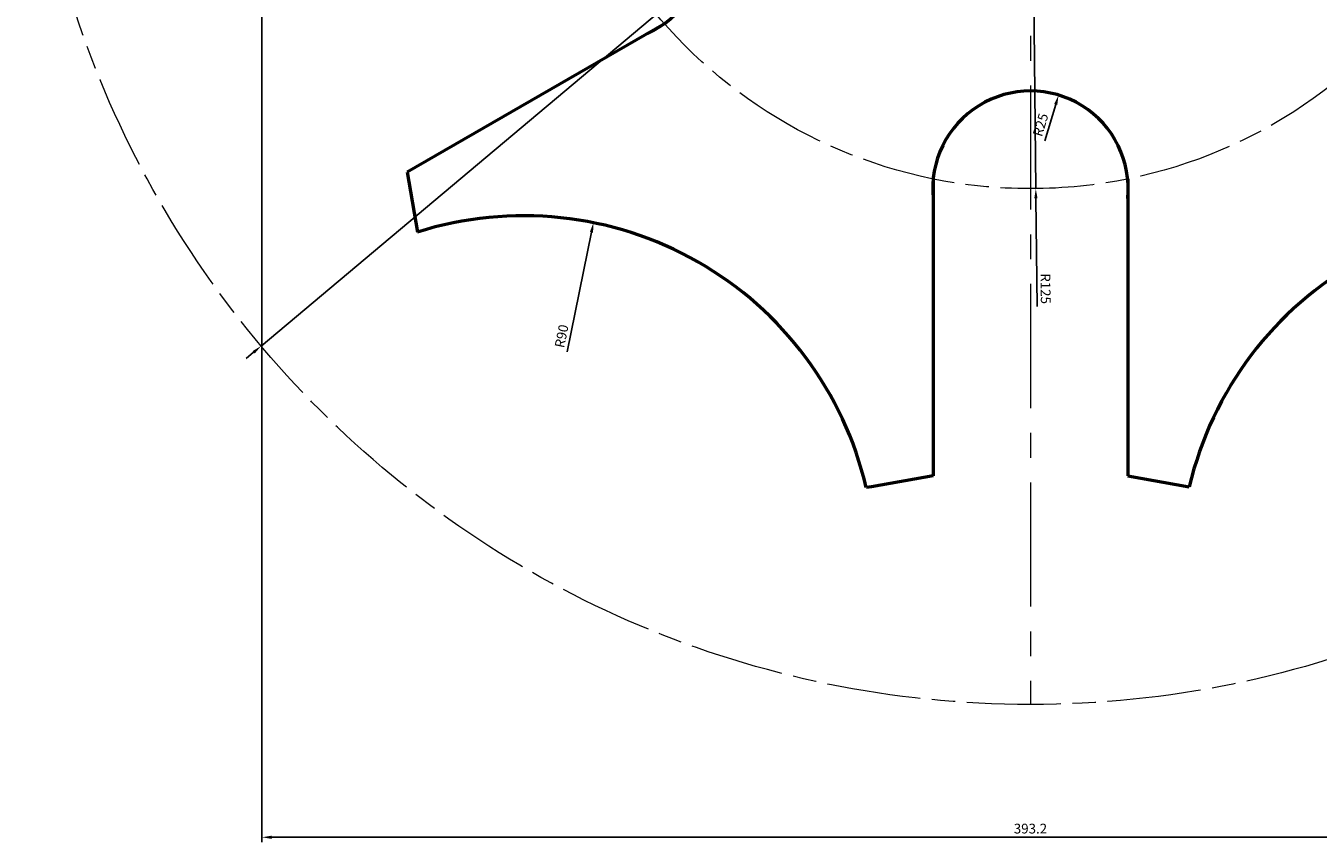
# Model space of a CAD drawing. Units: millimetres. Extents: x 1944 to 2645, y 1235 to 1798.
# Tile 1 of 3: x 2069 to 2400, y 1235 to 1444. Entities that reach past the tile are written whole.
import ezdxf

# ---------------------------------------------------------------- set-up
doc = ezdxf.new("R2010")
doc.units = ezdxf.units.MM
doc.linetypes.add('ACAD_ISO08W100', pattern=[36, 24, -3, 6, -3])
doc.linetypes.add('CENTER', pattern=[50.8, 31.75, -6.35, 6.35, -6.35])
for name, color, linetype, lineweight in [('M-CNTR', 4, 'CENTER', 18), ('M-CONS', 8, 'ACAD_ISO08W100', 18), ('M-DIMS', 2, 'Continuous', 25), ('M-OUTL', 7, 'Continuous', 50)]:
    doc.layers.add(name, color=color, linetype=linetype, lineweight=lineweight)
doc.styles.get("Standard").update_dxf_attribs({"font": 'arial.ttf'})
doc.dimstyles.new('ISO-25', dxfattribs={"dimtxt": 2.5, "dimasz": 2.5, "dimexe": 1.25, "dimexo": 0.625, "dimtad": 1, "dimdec": 1, "dimdsep": 46, "dimtxsty": 'Standard', "dimcen": 2.5, "dimadec": 0, "dimazin": 0, "dimtfac": 1, "dimtdec": 1, "dimtmove": 0, "dimatfit": 3, "dimfxl": 1, "dimarcsym": 0})

# ---------------------------------------------------------------- blocks, each defined once
blk = doc.blocks.new('*D3')
at = {"layer": 'Defpoints', "color": 0, "lineweight": 100, "transparency": 16777216}
for p in [(2333.34, 1426.64), (2326.15, 1402.69)]:
    blk.add_point(p, dxfattribs=at)
at = {"layer": 'M-DIMS', "color": 0, "lineweight": -2, "transparency": 16777216}
blk.add_line((2329.82, 1414.91), (2332.62, 1424.24), dxfattribs=at)
at = {"layer": 'M-DIMS', "color": 0, "lineweight": 100, "transparency": 16777216}
blk.add_solid([(2332.22, 1424.36), (2333.02, 1424.12), (2333.34, 1426.64)], dxfattribs=at)
at = {"layer": 'M-DIMS', "color": 0, "transparency": 16777216, "insert": (2329.04, 1418.93), "char_height": 2.5, "attachment_point": 5, "rotation": 73.2857}
blk.add_mtext('R25', dxfattribs=at)
blk = doc.blocks.new('*D6')
at = {"layer": 'Defpoints', "color": 0, "lineweight": 100, "transparency": 16777216}
for p in [(2326.15, 1527.69), (2327.52, 1402.7)]:
    blk.add_point(p, dxfattribs=at)
at = {"layer": 'M-DIMS', "color": 0, "lineweight": -2, "transparency": 16777216}
for p, q in [((2326.15, 1527.69), (2327.52, 1402.7)), ((2327.85, 1372.49), (2327.55, 1400.2))]:
    blk.add_line(p, q, dxfattribs=at)
at = {"layer": 'M-DIMS', "color": 0, "lineweight": 100, "transparency": 16777216}
blk.add_solid([(2327.96, 1400.2), (2327.13, 1400.19), (2327.52, 1402.7)], dxfattribs=at)
at = {"layer": 'M-DIMS', "color": 0, "transparency": 16777216, "insert": (2329.7, 1377.1), "char_height": 2.5, "attachment_point": 5, "rotation": 270.6275}
blk.add_mtext('R125', dxfattribs=at)
blk = doc.blocks.new('*D7')
at = {"layer": 'Defpoints', "color": 0, "lineweight": 100, "transparency": 16777216}
for p in [(2214.35, 1393.97), (2196.48, 1305.76)]:
    blk.add_point(p, dxfattribs=at)
at = {"layer": 'M-DIMS', "color": 0, "lineweight": -2, "transparency": 16777216}
blk.add_line((2207.66, 1360.97), (2213.85, 1391.52), dxfattribs=at)
at = {"layer": 'M-DIMS', "color": 0, "lineweight": 100, "transparency": 16777216}
blk.add_solid([(2213.44, 1391.6), (2214.26, 1391.44), (2214.35, 1393.97)], dxfattribs=at)
at = {"layer": 'M-DIMS', "color": 0, "transparency": 16777216, "insert": (2206.52, 1364.88), "char_height": 2.5, "attachment_point": 5, "rotation": 78.5527}
blk.add_mtext('R90', dxfattribs=at)
blk = doc.blocks.new('*D13')
at = {"layer": 'Defpoints', "color": 0, "lineweight": 100, "transparency": 16777216}
for p in [(2160.02, 1723.78), (2492.28, 1331.61)]:
    blk.add_point(p, dxfattribs=at)
at = {"layer": 'M-DIMS', "color": 0, "lineweight": -2, "transparency": 16777216}
blk.add_line((2467.27, 1361.13), (2490.67, 1333.51), dxfattribs=at)
at = {"layer": 'M-DIMS', "color": 0, "lineweight": 100, "transparency": 16777216}
blk.add_solid([(2490.98, 1333.78), (2490.35, 1333.24), (2492.28, 1331.61)], dxfattribs=at)
at = {"layer": 'M-DIMS', "color": 0, "transparency": 16777216, "insert": (2471.84, 1358.79), "char_height": 2.5, "attachment_point": 5, "rotation": 310.2727}
blk.add_mtext('∅514', dxfattribs=at)
blk = doc.blocks.new('GENEVA-RADIAL-SLOT-R25')
for p, q in [((0.13, 76), (0.13, 0)), ((49.87, 76), (49.87, 0))]:
    blk.add_line(p, q)
blk.add_arc((25, 73.5), 25, 354.2608, 185.7392)
blk = doc.blocks.new('*D17')
at = {"layer": 'Defpoints', "color": 0, "lineweight": 100, "transparency": 16777216}
for p in [(2129.55, 1460.27), (2522.75, 1460.27), (2522.75, 1236.69)]:
    blk.add_point(p, dxfattribs=at)
at = {"layer": 'M-DIMS', "color": 0, "lineweight": -2, "transparency": 16777216}
for p, q in [((2129.55, 1459.64), (2129.55, 1235.44)), ((2522.75, 1459.64), (2522.75, 1235.44)), ((2132.05, 1236.69), (2520.25, 1236.69))]:
    blk.add_line(p, q, dxfattribs=at)
at = {"layer": 'M-DIMS', "color": 0, "lineweight": 100, "transparency": 16777216}
for points in [[(2132.05, 1237.11), (2132.05, 1236.27), (2129.55, 1236.69)], [(2520.25, 1237.11), (2520.25, 1236.27), (2522.75, 1236.69)]]:
    blk.add_solid(points, dxfattribs=at)
at = {"layer": 'M-DIMS', "color": 0, "transparency": 16777216, "insert": (2326.15, 1238.59), "char_height": 2.5, "attachment_point": 5}
blk.add_mtext('393.2', dxfattribs=at)
blk = doc.blocks.new('*D18')
at = {"layer": 'Defpoints', "color": 0, "lineweight": 100, "transparency": 16777216}
for p in [(2522.96, 1692.97), (2129.34, 1362.42)]:
    blk.add_point(p, dxfattribs=at)
at = {"layer": 'M-DIMS', "color": 0, "lineweight": -2, "transparency": 16777216}
for p, q in [((2644.67, 1795.18), (2524.87, 1694.57)), ((2129.34, 1362.42), (2522.96, 1692.97)), ((2127.43, 1360.81), (2125.51, 1359.2))]:
    blk.add_line(p, q, dxfattribs=at)
at = {"layer": 'M-DIMS', "color": 0, "lineweight": 100, "transparency": 16777216}
for points in [[(2524.61, 1694.89), (2525.14, 1694.25), (2522.96, 1692.97)], [(2127.16, 1361.13), (2127.69, 1360.49), (2129.34, 1362.42)]]:
    blk.add_solid(points, dxfattribs=at)
at = {"layer": 'M-DIMS', "color": 0, "transparency": 16777216, "insert": (2639.78, 1793.64), "char_height": 2.5, "attachment_point": 5, "rotation": 40.0225}
blk.add_mtext('∅514', dxfattribs=at)

msp = doc.modelspace()

# ---------------------------------------------------------------- linework, layer by layer
at = {"layer": 'M-CNTR'}
msp.add_line((2326.15, 1784.69), (2326.15, 1270.69), dxfattribs=at)
at = {"layer": 'M-CONS'}
for radius in [257, 125]:
    msp.add_circle((2326.15, 1527.69), radius, dxfattribs=at)
at = {"layer": 'M-OUTL'}
for p, q in [((2166.68, 1406.9), (2169.38, 1391.58)), ((2301.28, 1329.19), (2285.52, 1326.41)), ((2351.02, 1329.19), (2366.78, 1326.41)), ((2285.52, 1326.41), (2284.14, 1326.17))]:
    msp.add_line(p, q, dxfattribs=at)
for centre, start, end in [((2196.48, 1305.76), 13.1069, 107.526), ((2454.38, 1305.76), 71.5652, 166.7342)]:
    msp.add_arc(centre, 90, start, end, dxfattribs=at)

# ---------------------------------------------------------------- block references
at = {"layer": 'M-OUTL', "rotation": 300.0000000000004}
msp.add_blockref('GENEVA-RADIAL-SLOT-R25', (2141.74, 1450.09), dxfattribs=at)
at = {"layer": 'M-OUTL'}
msp.add_blockref('GENEVA-RADIAL-SLOT-R25', (2301.15, 1329.19), dxfattribs=at)

# ---------------------------------------------------------------- dimensions: what is measured, and where the dimension line sits
at = {"layer": 'M-DIMS'}
for p1, p2, override, picture, middle in [((2129.34, 1362.42), (2522.96, 1692.97), {"dimdec": 0, "dimlfac": 1, "dimrnd": 0, "dimzin": 0, "dimdsep": 46, "dimlunit": 2}, '*D18', (2641.04, 1792.13)), ((2160.02, 1723.78), (2492.28, 1331.61), {"dimclrd": 0, "dimclre": 0, "dimclrt": 0}, '*D13', (2470.33, 1357.51))]:
    dim = msp.add_diameter_dim_2p(p1=p1, p2=p2, dimstyle='ISO-25', override=override, dxfattribs=at)
    dim.commit()
    dim.dimension.update_dxf_attribs({"geometry": picture, "text_midpoint": middle, "dimtype": 163})
for center, mpoint, picture, middle in [((2326.15, 1527.69), (2327.52, 1402.7), '*D6', (2327.8, 1377.08)), ((2326.15, 1402.69), (2333.34, 1426.64), '*D3', (2330.86, 1418.38)), ((2196.48, 1305.76), (2214.35, 1393.97), '*D7', (2208.38, 1364.5))]:
    dim = msp.add_radius_dim(center=center, mpoint=mpoint, dimstyle='ISO-25', override={"dimclrd": 0, "dimclre": 0, "dimclrt": 0}, dxfattribs=at)
    dim.commit()
    dim.dimension.update_dxf_attribs({"geometry": picture, "text_midpoint": middle, "dimtype": 164})
dim = msp.add_linear_dim(base=(2522.75, 1236.69), p1=(2129.55, 1460.27), p2=(2522.75, 1460.27), dimstyle='ISO-25', override={"dimdec": 1, "dimlfac": 1, "dimrnd": 0, "dimzin": 0, "dimdsep": 46, "dimlunit": 2}, dxfattribs=at)
dim.commit()
dim.dimension.update_dxf_attribs({"geometry": '*D17', "text_midpoint": (2326.15, 1238.59)})

doc.saveas('drawing.dxf')
